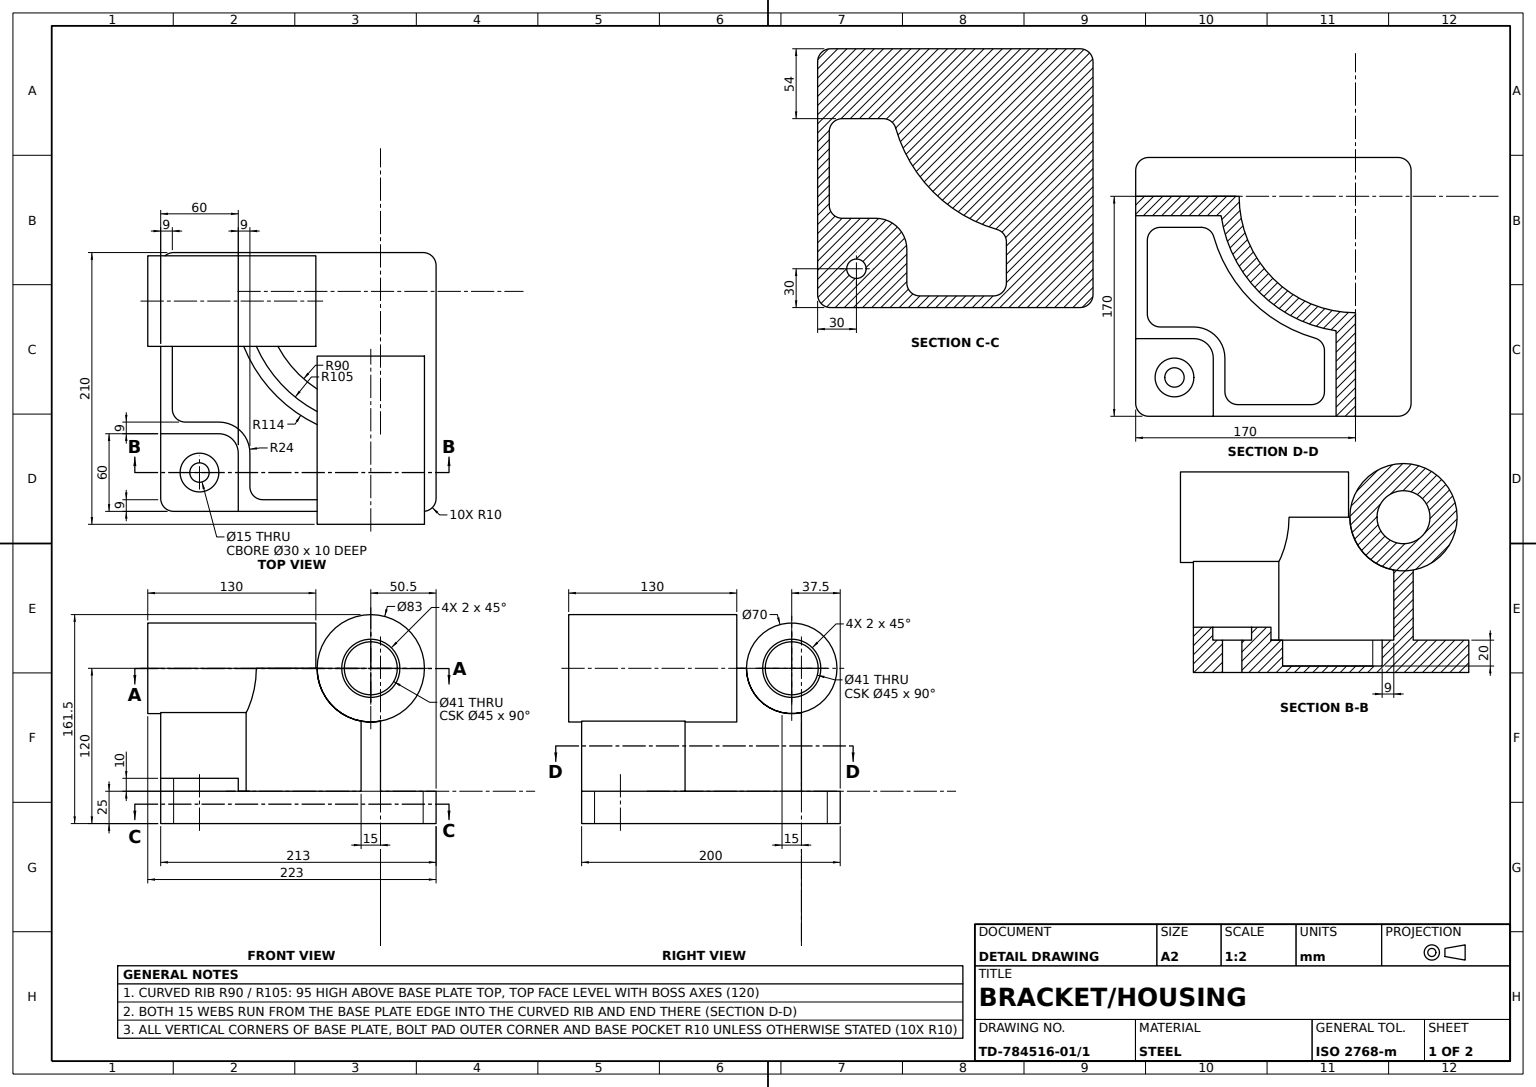
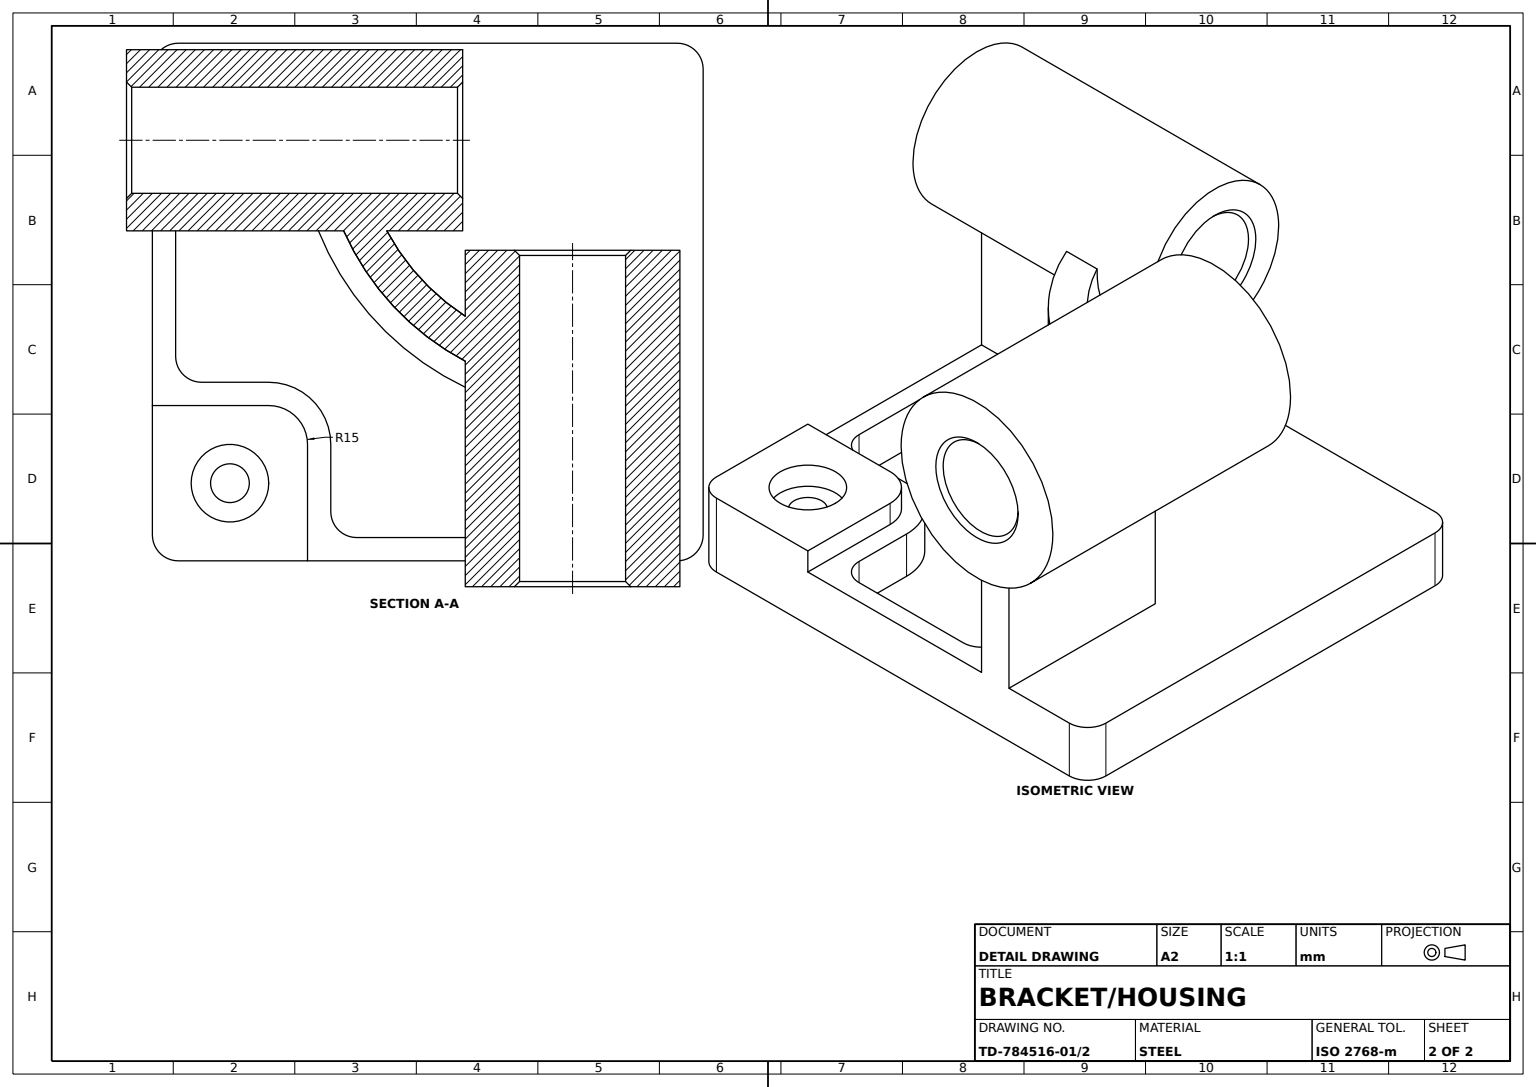
SolidWorks part; units mm, degrees
material "Plain Carbon Steel"
ref_plane "Front Plane" through (0, 0, 0) normal (0, 0, 1) x (1, 0, 0)
ref_plane "Top Plane" through (0, 0, 0) normal (0, 1, 0) x (1, 0, 0)
ref_plane "Right Plane" through (0, 0, 0) normal (1, 0, 0) x (0, 0, -1)
sketch "Base Plate Sketch" plane through (0, 0, 0) normal (0, 1, 0) x (1, 0, 0)
  line L1 (-100, -106.5) -> (100, -106.5)
  line L2 (-100, -106.5) -> (-100, 106.5)
  line L3 (-100, 106.5) -> (100, 106.5)
  line L4 (100, -106.5) -> (100, 106.5)
  line L5 (-100, -106.5) -> (100, 106.5) construction
  line L6 (-100, 106.5) -> (100, -106.5) construction
  point P0 (0, 0)
  dimension "D1" = 213
  dimension "D2" = 200
extrude "Base Plate" add sketch "Base Plate Sketch" along normal blind 25
sketch "Bolt Pad Sketch" plane through (0, 25, 0) normal (0, 1, 0) x (1, 0, 0)
  line L1 (100, -106.5) -> (40, -106.5)
  line L2 (100, -106.5) -> (100, -46.5)
  line L3 (100, -46.5) -> (55, -46.5)
  line L4 (40, -106.5) -> (40, -61.5)
  arc A0 (55, -46.5) -> (40, -61.5) centre (55, -61.5) ccw
  dimension "D2" = 15
  dimension "D1" = 60
extrude "Bolt Pad" add sketch "Bolt Pad Sketch" along normal blind 10
fillet "Base Plate Fillets R10" radius 10 4 edges at (100, 12.5, -106.5) (-100, 12.5, -106.5) (100, 17.5, 106.5) (-100, 12.5, 106.5)
sketch "Central Housing Sketch" plane through (0, 25, 0) normal (0, 1, 0) x (1, 0, 0)
  line L0 (-100, 63.5) -> (100, 63.5) construction
  line L1 (-100, 96.5) -> (-100, -96.5) construction
  line L2 (100, -46.5) -> (100, 96.5) construction
  line L3 (-70, 106.5) -> (-70, -106.5) construction
  line L4 (90, 106.5) -> (-90, 106.5) construction
  line L5 (-90, -106.5) -> (40, -106.5) construction
  line L6 (100, 63.5) -> (20, 63.5)
  line L7 (-70, -26.5) -> (-70, -106.5)
  line L8 (100, 48.5) -> (33.923, 48.5)
  line L9 (-55, -40.423) -> (-55, -106.5)
  line L10 (-70, -106.5) -> (-55, -106.5)
  line L11 (100, 48.5) -> (100, 63.5)
  arc A0 (20, 63.5) -> (-70, -26.5) centre (-70, 63.5) cw
  arc A1 (33.923, 48.5) -> (-55, -40.423) centre (-70, 63.5) cw
  dimension "D3" = 80
  dimension "D4" = 15
  dimension "D1" = 170
  dimension "D2" = 170
extrude "Central Housing" add sketch "Central Housing Sketch" along normal blind 95
sketch "Bearing Boss A Sketch" plane through (0, 0, 106.5) normal (0, 0, 1) x (1, 0, 0)
  line L0 (-70, 120) -> (-55, 120) construction
  circle A0 centre (-62.5, 120) radius 35
  dimension "D1" = 70
extrude "Bearing Boss A" add sketch "Bearing Boss A Sketch" along normal blind 10 and the other way blind 120
sketch "Bearing Boss B Sketch" plane through (100, 0, 0) normal (1, 0, 0) x (0, 0, -1)
  line L0 (48.5, 120) -> (63.5, 120) construction
  circle A0 centre (56, 120) radius 41.5
  dimension "D1" = 83
extrude "Bearing Boss B" add sketch "Bearing Boss B Sketch" along normal blind 10 and the other way blind 120
sketch "Bearing Bore A Sketch" plane through (0, 0, 116.5) normal (0, 0, 1) x (1, 0, 0)
  circle A0 centre (-62.5, 120) radius 20.5
  dimension "D1" = 41
extrude "Bearing Bore A Ø41" cut sketch "Bearing Bore A Sketch" against normal up to next
sketch "Bearing Bore B Sketch" plane through (110, 0, 0) normal (1, 0, 0) x (0, 0, -1)
  circle A0 centre (56, 120) radius 20.5
  dimension "D1" = 41
extrude "Bearing Bore B Ø41" cut sketch "Bearing Bore B Sketch" against normal up to next
chamfer "Bore Chamfers 2x45°" distance 2 angle 45 4 edges at (-42, 120, -13.5) (-42, 120, 116.5) (-20, 120, -76.5) (110, 120, -76.5)
hole_wizard "M8 Counterbored Mounting Hole" positions "3DSketch1" profile "Sketch11" counterbore size "M8" standard "ANSI Metric" end condition through all
sketch3d "3DSketch1"
  line L0 (100, 35, 46.5) -> (55, 35, 46.5) construction
  line L1 (40, 35, 61.5) -> (40, 35, 106.5) construction
  point P0 (70, 35, 76.5)
  dimension "D1" = 30
  dimension "D2" = 30
sketch "Sketch11" plane through (70, 35, 76.5) normal (1, 0, 0) x (0, 0, 1)
  line L0 (0, 0) -> (0, 35)
  line L1 (0, 35) -> (7.5, 35)
  line L3 (7.5, 35) -> (7.5, 10)
  line L4 (7.5, 10) -> (15, 10)
  line L5 (15, 10) -> (15, 0)
  line L7 (15, 0) -> (0, 0)
  line L11 (0, -6.35) -> (0, 107.95) construction
  dimension "Thru Hole Dia." = 15
  dimension "Thru Hole Depth" = 35
  dimension "C'Bore Dia." = 30
  dimension "C'Bore Depth" = 10
sketch "Base Pocket Sketch" plane through (0, 25, 0) normal (0, 1, 0) x (1, 0, 0)
  line L12 (-46, -47.9451) -> (-46, -97.5)
  line L13 (-46, -97.5) -> (31, -97.5)
  line L14 (31, -97.5) -> (31, -61.5)
  line L15 (55, -37.5) -> (91, -37.5)
  line L16 (91, -37.5) -> (91, 39.5)
  line L17 (91, 39.5) -> (41.4451, 39.5)
  line L18 (-46, -55.7476) -> (-46, -87.5)
  line L19 (-36, -97.5) -> (21, -97.5)
  line L20 (31, -87.5) -> (31, -61.5)
  line L21 (55, -37.5) -> (81, -37.5)
  line L22 (91, -27.5) -> (91, 29.5)
  line L23 (81, 39.5) -> (49.2476, 39.5)
  arc A2 (-46, -55.7476) -> (-38.7419, -46.1309) centre (-36, -55.7476) cw
  arc A3 (-46, -87.5) -> (-36, -97.5) centre (-36, -87.5) ccw
  arc A4 (55, -37.5) -> (31, -61.5) centre (55, -61.5) ccw
  arc A5 (-46, -47.9451) -> (41.4451, 39.5) centre (-70, 63.5) ccw
  arc A6 (55, -37.5) -> (31, -61.5) centre (55, -61.5) ccw
  arc A7 (-38.7419, -46.1309) -> (39.6309, 32.2419) centre (-70, 63.5) ccw
  arc A8 (21, -97.5) -> (31, -87.5) centre (21, -87.5) ccw
  arc A9 (81, -37.5) -> (91, -27.5) centre (81, -27.5) ccw
  arc A10 (91, 29.5) -> (81, 39.5) centre (81, 29.5) ccw
  arc A11 (49.2476, 39.5) -> (39.6309, 32.2419) centre (49.2476, 29.5) ccw
  dimension "D2" = 10
  dimension "D1" = 9
extrude "Base Pocket" cut sketch "Base Pocket Sketch" against normal blind 20
